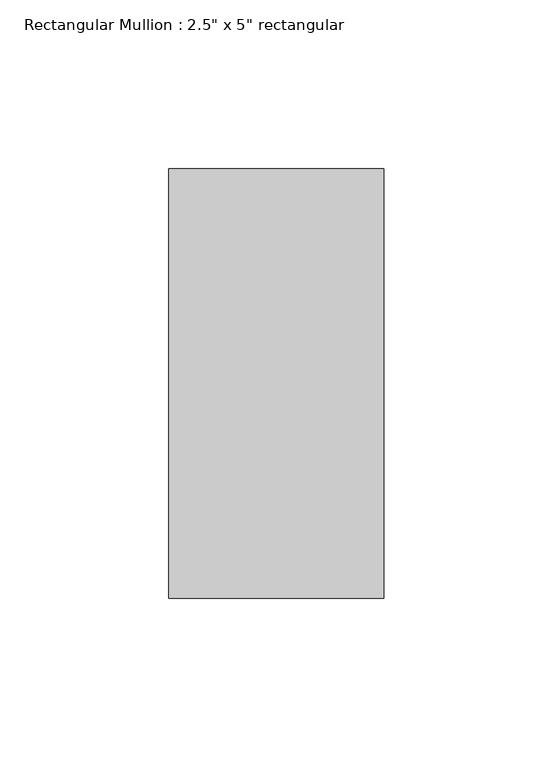
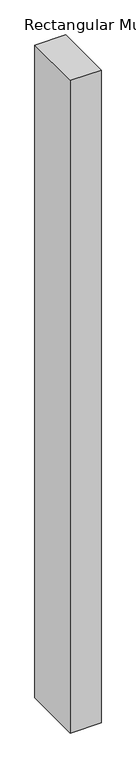
"""IFC4 building model written with IfcOpenShell, lengths in millimetres: member geometry."""

from ifc_helpers import new_model, si_unit, frame, origin, place, context, project, spatial, polyline, outline, extrude, source, transform, mapped, element, save


def member_2e265c97(model_context):
    return source(origin(), model_context, "Body", "SweptSolid", [
        extrude(outline(polyline([(31.75, 63.5), (31.75, -63.5), (-31.75, -63.5), (-31.75, 63.5), (31.75, 63.5)])), frame((0.0, 0.0, -1428.7500001), z_axis=(0.0, 0.0, 1.0), x_axis=(1.0, 0.0, 0.0)), (0.0, 0.0, 1.0), 1428.7500001),
    ])


if __name__ == "__main__":
    model = new_model("IFC4")
    model_context = context("Model", 3, world=origin())
    ifc_project = project(units=[si_unit("LENGTHUNIT", "METRE", prefix="MILLI")], contexts=[model_context])
    site = spatial("IfcSite", under=ifc_project)
    building = spatial("IfcBuilding", under=site)
    placement = place(None, origin())
    member_shape = member_2e265c97(model_context)
    element("IfcMember", 1, ObjectType="Rectangular Mullion : 2.5\" x 5\" rectangular", at=placement, inside=building, context=model_context, shape_type="MappedRepresentation", body=[
        mapped(member_shape, transform((0.0, 0.0, 0.0), x_axis=(1.0, 0.0, 0.0), y_axis=(0.0, 1.0, 0.0), z_axis=(0.0, 0.0, 1.0))),
    ])
    save(model, "model.ifc")

# Revit data of these elements
# Type "Rectangular Mullion : 2.5\" x 5\" rectangular"
#   built-in parameter 1007304 = 0.416667 (stored number, unit not read)
#   built-in parameter 1007301 = 0.104167 (stored number, unit not read)
#   built-in parameter 1007300 = 0.104167 (stored number, unit not read)
# Element 1 (IfcMember, "Rectangular Mullion : 2.5\" x 5\" rectangular")
#   Materials on its faces: "BLACK COLOUR"
# Materials
#   "BLACK COLOUR": class "Generic", colour RGB 120 120 120, transparency 0, Cost = 0
